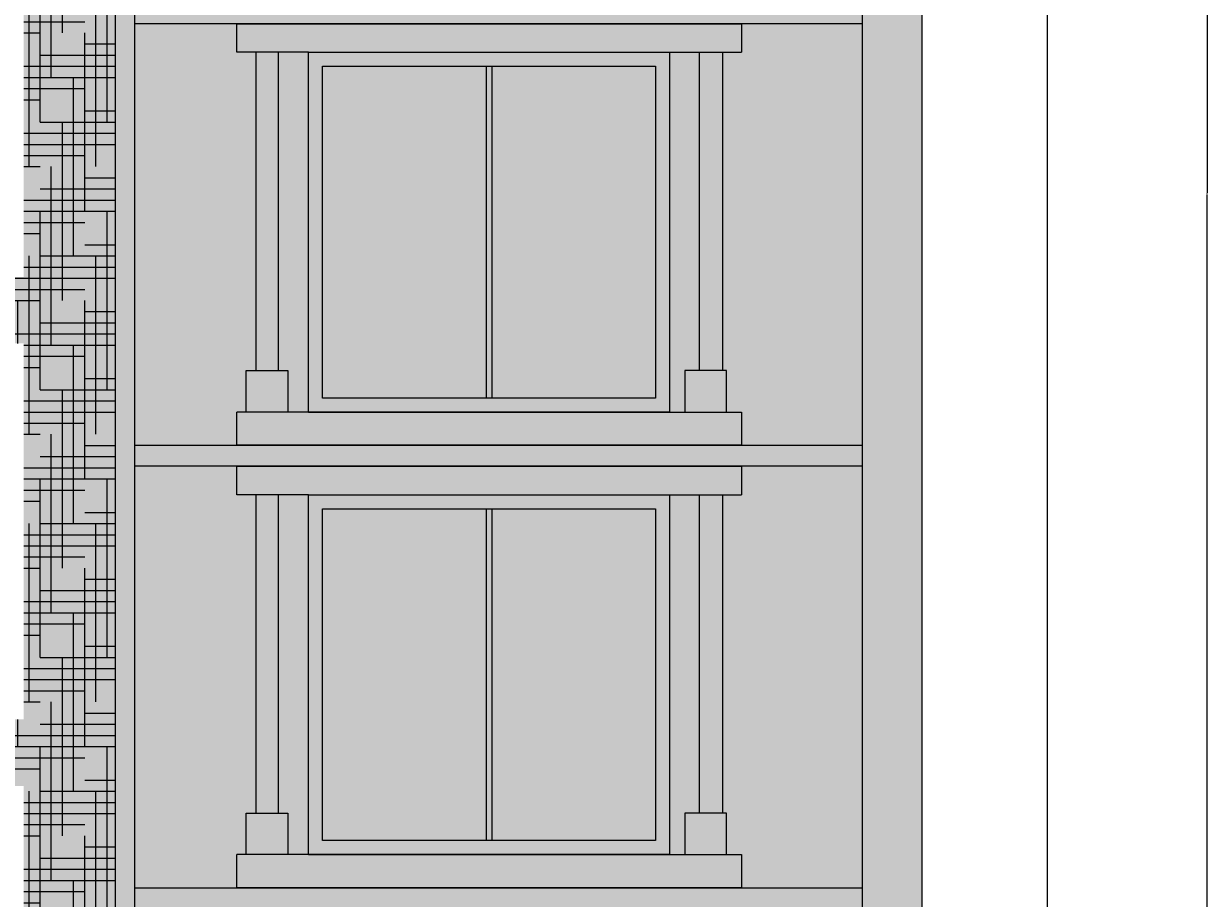
# Model space of a CAD drawing. Units: inches. Extents: x 3024 to 4744, y 1110 to 2100.
# Tile 17 of 29: x 3450 to 3787, y 1405 to 1654. Entities that reach past the tile are written whole.
import ezdxf

# ---------------------------------------------------------------- set-up
doc = ezdxf.new("R2010")
doc.units = ezdxf.units.IN
for name, color, linetype, lineweight in [('A-ANNO-DIMS', 2, 'Continuous', 18), ('A-ELEV', 7, 'Continuous', 25), ('A-ELEV-PATT', 252, 'Continuous', 13), ('A-GLAZ', 4, 'Continuous', 18)]:
    doc.layers.add(name, color=color, linetype=linetype, lineweight=lineweight)
doc.styles.get("Standard").update_dxf_attribs({"font": 'arial.ttf'})
doc.dimstyles.get("Standard").update_dxf_attribs({"dimtxt": 0.18, "dimasz": 0.18, "dimexe": 0.18, "dimexo": 0.0625, "dimgap": 0.09, "dimtad": 0, "dimtih": 1, "dimtoh": 1, "dimdec": 1, "dimzin": 0, "dimdsep": 46, "dimlunit": 3, "dimtxsty": 'Standard', "dimcen": 0.09, "dimadec": 0, "dimazin": 0, "dimtfac": 1, "dimtdec": 1, "dimtofl": 0, "dimtmove": 0, "dimatfit": 3, "dimfxl": 1, "dimtolj": 1, "dimtzin": 0, "dimarcsym": 0})

# ---------------------------------------------------------------- blocks, each defined once
blk = doc.blocks.new('WIN-BALCONY-A')
for p, q in [((3169.4, 1897.49), (3148.97, 1897.49)), ((3169.4, 1897.49), (3148.97, 1897.49)), ((3169.4, 1897.49), (3292.61, 1897.49)), ((3169.4, 1897.49), (3292.61, 1897.49)), ((3169.4, 1795.04), (3148.97, 1795.04)), ((3169.4, 1795.04), (3148.97, 1795.04)), ((3169.4, 1795.04), (3292.61, 1795.04)), ((3169.4, 1795.04), (3292.61, 1795.04))]:
    blk.add_line(p, q)
for points in [[(3148.97, 1897.49), (3148.97, 1905.61), (3292.61, 1905.61), (3292.61, 1897.49)], [(3148.97, 1897.49), (3148.97, 1905.61), (3292.61, 1905.61), (3292.61, 1897.49)], [(3292.61, 1795.04), (3292.61, 1785.61), (3148.97, 1785.61), (3148.97, 1795.04)], [(3292.61, 1795.04), (3292.61, 1785.61), (3148.97, 1785.61), (3148.97, 1795.04)]]:
    blk.add_lwpolyline(points)
for points in [[(3154.33, 1806.87), (3160.86, 1806.87), (3160.86, 1897.49), (3154.33, 1897.49)], [(3154.33, 1806.87), (3160.86, 1806.87), (3160.86, 1897.49), (3154.33, 1897.49)], [(3272.18, 1795.04), (3169.4, 1795.04), (3169.4, 1897.49), (3272.18, 1897.49)], [(3272.18, 1795.04), (3169.4, 1795.04), (3169.4, 1897.49), (3272.18, 1897.49)], [(3287.25, 1806.87), (3280.72, 1806.87), (3280.72, 1897.49), (3287.25, 1897.49)], [(3287.25, 1806.87), (3280.72, 1806.87), (3280.72, 1897.49), (3287.25, 1897.49)], [(3268.18, 1799.04), (3173.4, 1799.04), (3173.4, 1893.49), (3268.18, 1893.49)], [(3268.18, 1799.04), (3173.4, 1799.04), (3173.4, 1893.49), (3268.18, 1893.49)], [(3220.05, 1893.49), (3221.52, 1893.49), (3221.52, 1799.04), (3220.05, 1799.04)], [(3220.05, 1893.49), (3221.52, 1893.49), (3221.52, 1799.04), (3220.05, 1799.04)], [(3163.53, 1795.04), (3151.66, 1795.04), (3151.66, 1806.87), (3163.53, 1806.87)], [(3163.53, 1795.04), (3151.66, 1795.04), (3151.66, 1806.87), (3163.53, 1806.87)], [(3276.51, 1795.04), (3288.38, 1795.04), (3288.38, 1806.87), (3276.51, 1806.87)], [(3276.51, 1795.04), (3288.38, 1795.04), (3288.38, 1806.87), (3276.51, 1806.87)]]:
    blk.add_lwpolyline(points, close=True)
blk = doc.blocks.new('*D64')
at = {"layer": 'A-ANNO-DIMS', "color": 0, "lineweight": -2, "transparency": 16777216}
for p, q in [((3069.79, 1241.5), (3069.79, 2100.44)), ((3069.97, 2100.26), (3405.08, 2100.26)), ((3740.97, 2100.26), (3405.87, 2100.26)), ((3741.15, 1241.5), (3741.15, 2100.44))]:
    blk.add_line(p, q, dxfattribs=at)
at = {"layer": 'A-ANNO-DIMS', "color": 0, "transparency": 16777216}
for points in [[(3069.97, 2100.29), (3069.97, 2100.23), (3069.79, 2100.26)], [(3740.97, 2100.29), (3740.97, 2100.23), (3741.15, 2100.26)]]:
    blk.add_solid(points, dxfattribs=at)
at = {"layer": 'Defpoints', "color": 0, "transparency": 16777216}
for p in [(3741.15, 2100.26), (3069.79, 1241.43), (3741.15, 1241.43)]:
    blk.add_point(p, dxfattribs=at)
at = {"layer": 'A-ANNO-DIMS', "color": 0, "transparency": 16777216, "insert": (3405.47, 2100.26), "char_height": 0.18, "attachment_point": 5}
blk.add_mtext('\\A1;671.4', dxfattribs=at)
blk = doc.blocks.new('*D75')
at = {"layer": 'A-ANNO-DIMS', "color": 0, "lineweight": -2, "transparency": 16777216}
for p, q in [((3491.89, 2054.76), (3786.83, 2054.76)), ((3786.65, 2054.58), (3786.65, 1605.37)), ((3786.65, 1155.79), (3786.65, 1605)), ((3741.21, 1155.61), (3786.83, 1155.61))]:
    blk.add_line(p, q, dxfattribs=at)
at = {"layer": 'A-ANNO-DIMS', "color": 0, "transparency": 16777216}
for points in [[(3786.62, 2054.58), (3786.68, 2054.58), (3786.65, 2054.76)], [(3786.62, 1155.79), (3786.68, 1155.79), (3786.65, 1155.61)]]:
    blk.add_solid(points, dxfattribs=at)
at = {"layer": 'Defpoints', "color": 0, "transparency": 16777216}
for p in [(3491.83, 2054.76), (3786.65, 2054.76), (3741.15, 1155.61)]:
    blk.add_point(p, dxfattribs=at)
at = {"layer": 'A-ANNO-DIMS', "color": 0, "transparency": 16777216, "insert": (3786.65, 1605.18), "char_height": 0.18, "attachment_point": 5}
blk.add_mtext('\\A1;899.1', dxfattribs=at)

msp = doc.modelspace()

# ---------------------------------------------------------------- hatches: boundary and pattern name
at = {"layer": 'A-ELEV-PATT'}
h = msp.add_hatch(color=256, dxfattribs=at)
h.dxf.hatch_style = 1
h.paths.add_polyline_path([(3491.8271, 2054.7584), (3320.5658, 2054.7584), (3320.5658, 2043.5286), (3491.8271, 2043.5286)])
h.paths.add_polyline_path([(3292.6051, 1905.6112), (3148.9694, 1905.6112), (3148.9694, 1897.4879), (3169.3964, 1897.4879), (3292.6051, 1897.4879)])
h.paths.add_polyline_path([(3292.6051, 1795.0431), (3169.3964, 1795.0431), (3148.9694, 1795.0431), (3148.9694, 1785.6112), (3292.6051, 1785.6112)])
h.paths.add_polyline_path([(3292.6051, 1779.6112), (3148.9694, 1779.6112), (3148.9694, 1771.4879), (3169.3964, 1771.4879), (3292.6051, 1771.4879)])
h.paths.add_polyline_path([(3292.6051, 1669.0431), (3169.3964, 1669.0431), (3148.9694, 1669.0431), (3148.9694, 1659.6112), (3292.6051, 1659.6112)])
h.paths.add_polyline_path([(3292.6051, 1653.6112), (3148.9694, 1653.6112), (3148.9694, 1645.4879), (3169.3964, 1645.4879), (3292.6051, 1645.4879)])
h.paths.add_polyline_path([(3292.6051, 1543.0431), (3169.3964, 1543.0431), (3148.9694, 1543.0431), (3148.9694, 1533.6112), (3292.6051, 1533.6112)])
h.paths.add_polyline_path([(3292.6051, 1527.6112), (3148.9694, 1527.6112), (3148.9694, 1519.4879), (3169.3964, 1519.4879), (3292.6051, 1519.4879)])
h.paths.add_polyline_path([(3292.6051, 1401.6112), (3148.9694, 1401.6112), (3148.9694, 1393.4879), (3169.3964, 1393.4879), (3292.6051, 1393.4879)])
h.paths.add_polyline_path([(3292.6051, 1417.0431), (3169.3964, 1417.0431), (3148.9694, 1417.0431), (3148.9694, 1407.6112), (3292.6051, 1407.6112)])
h.paths.add_polyline_path([(3292.6051, 1291.0431), (3169.3964, 1291.0431), (3148.9694, 1291.0431), (3148.9694, 1281.6112), (3292.6051, 1281.6112)])
h.paths.add_polyline_path([(3654.037, 1165.0431), (3530.8283, 1165.0431), (3510.4013, 1165.0431), (3510.4013, 1155.6112), (3654.037, 1155.6112)])
h.paths.add_polyline_path([(3654.037, 1275.6112), (3510.4013, 1275.6112), (3510.4013, 1267.4879), (3530.8283, 1267.4879), (3654.037, 1267.4879)])
h.paths.add_polyline_path([(3654.037, 1291.0431), (3530.8283, 1291.0431), (3510.4013, 1291.0431), (3510.4013, 1281.6112), (3654.037, 1281.6112)])
h.paths.add_polyline_path([(3654.037, 1417.0431), (3530.8283, 1417.0431), (3510.4013, 1417.0431), (3510.4013, 1407.6112), (3654.037, 1407.6112)])
h.paths.add_polyline_path([(3654.037, 1401.6112), (3510.4013, 1401.6112), (3510.4013, 1393.4879), (3530.8283, 1393.4879), (3654.037, 1393.4879)])
h.paths.add_polyline_path([(3654.037, 1543.0431), (3530.8283, 1543.0431), (3510.4013, 1543.0431), (3510.4013, 1533.6112), (3654.037, 1533.6112)])
h.paths.add_polyline_path([(3654.037, 1527.6112), (3510.4013, 1527.6112), (3510.4013, 1519.4879), (3530.8283, 1519.4879), (3654.037, 1519.4879)])
h.paths.add_polyline_path([(3654.037, 1653.6112), (3510.4013, 1653.6112), (3510.4013, 1645.4879), (3530.8283, 1645.4879), (3654.037, 1645.4879)])
h.paths.add_polyline_path([(3654.037, 1669.0431), (3530.8283, 1669.0431), (3510.4013, 1669.0431), (3510.4013, 1659.6112), (3654.037, 1659.6112)])
h.paths.add_polyline_path([(3654.037, 1779.6112), (3510.4013, 1779.6112), (3510.4013, 1771.4879), (3530.8283, 1771.4879), (3654.037, 1771.4879)])
h.paths.add_polyline_path([(3654.037, 1795.0431), (3530.8283, 1795.0431), (3510.4013, 1795.0431), (3510.4013, 1785.6112), (3654.037, 1785.6112)])
h.paths.add_polyline_path([(3654.037, 1905.6112), (3510.4013, 1905.6112), (3510.4013, 1897.4879), (3530.8283, 1897.4879), (3654.037, 1897.4879)])
h = msp.add_hatch(color=256, dxfattribs=at)
h.dxf.hatch_style = 1
h.paths.add_polyline_path([(3335.1044, 2043.5286), (3329.7033, 2043.5286), (3329.7033, 1155.6112), (3335.1044, 1155.6112)])
h.paths.add_polyline_path([(3481.2411, 2043.5286), (3335.1044, 2043.5286), (3335.1044, 1155.6112), (3481.2411, 1155.6112)])
h.paths.add_polyline_path([(3449.7202, 1329.5246), (3361.2242, 1329.5246), (3361.2242, 1436.6064), (3449.7202, 1436.6064)], flags=16)
h.paths.add_polyline_path([(3445.7202, 1333.5246), (3365.2242, 1333.5246), (3365.2242, 1432.6064), (3445.7202, 1432.6064)], flags=0)
h.paths.add_polyline_path([(3449.7202, 1455.5246), (3361.2242, 1455.5246), (3361.2242, 1562.6064), (3449.7202, 1562.6064)], flags=16)
h.paths.add_polyline_path([(3445.7202, 1459.5246), (3365.2242, 1459.5246), (3365.2242, 1558.6064), (3445.7202, 1558.6064)], flags=0)
h.paths.add_polyline_path([(3449.7202, 1581.5246), (3361.2242, 1581.5246), (3361.2242, 1688.6064), (3449.7202, 1688.6064)], flags=16)
h.paths.add_polyline_path([(3445.7202, 1585.5246), (3365.2242, 1585.5246), (3365.2242, 1684.6064), (3445.7202, 1684.6064)], flags=0)
h.paths.add_polyline_path([(3449.7202, 1707.5246), (3361.2242, 1707.5246), (3361.2242, 1814.6064), (3449.7202, 1814.6064)], flags=16)
h.paths.add_polyline_path([(3445.7202, 1711.5246), (3365.2242, 1711.5246), (3365.2242, 1810.6064), (3445.7202, 1810.6064)], flags=0)
h.paths.add_polyline_path([(3449.7202, 1833.5246), (3361.2242, 1833.5246), (3361.2242, 1940.6064), (3449.7202, 1940.6064)], flags=16)
h.paths.add_polyline_path([(3445.7202, 1837.5246), (3365.2242, 1837.5246), (3365.2242, 1936.6064), (3445.7202, 1936.6064)], flags=0)
h = msp.add_hatch(color=256, dxfattribs=at)
h.dxf.hatch_style = 1
h.paths.add_polyline_path([(3475.84, 2043.5286), (3335.1044, 2043.5286), (3335.1044, 1155.6112), (3475.84, 1155.6112)])
h.paths.add_polyline_path([(3449.7202, 1940.6064), (3449.7202, 1833.5246), (3361.2242, 1833.5246), (3361.2242, 1940.6064)], flags=16)
h.paths.add_polyline_path([(3445.7202, 1936.6064), (3445.7202, 1837.5246), (3365.2242, 1837.5246), (3365.2242, 1936.6064)], flags=0)
h.paths.add_polyline_path([(3449.7202, 1814.6064), (3449.7202, 1707.5246), (3361.2242, 1707.5246), (3361.2242, 1814.6064)], flags=16)
h.paths.add_polyline_path([(3445.7202, 1810.6064), (3445.7202, 1711.5246), (3365.2242, 1711.5246), (3365.2242, 1810.6064)], flags=0)
h.paths.add_polyline_path([(3449.7202, 1688.6064), (3449.7202, 1581.5246), (3361.2242, 1581.5246), (3361.2242, 1688.6064)], flags=16)
h.paths.add_polyline_path([(3445.7202, 1684.6064), (3445.7202, 1585.5246), (3365.2242, 1585.5246), (3365.2242, 1684.6064)], flags=0)
h.paths.add_polyline_path([(3449.7202, 1562.6064), (3449.7202, 1455.5246), (3361.2242, 1455.5246), (3361.2242, 1562.6064)], flags=16)
h.paths.add_polyline_path([(3445.7202, 1558.6064), (3445.7202, 1459.5246), (3365.2242, 1459.5246), (3365.2242, 1558.6064)], flags=0)
h.paths.add_polyline_path([(3449.7202, 1436.6064), (3449.7202, 1329.5246), (3361.2242, 1329.5246), (3361.2242, 1436.6064)], flags=16)
h.paths.add_polyline_path([(3445.7202, 1432.6064), (3445.7202, 1333.5246), (3365.2242, 1333.5246), (3365.2242, 1432.6064)], flags=0)
h = msp.add_hatch(dxfattribs=at)
h.set_pattern_fill('HOUND', color=256, scale=2)
h.paths.add_polyline_path([(3475.84, 2043.5286), (3335.1044, 2043.5286), (3335.1044, 1155.6112), (3475.84, 1155.6112)])
h.paths.add_polyline_path([(3449.7202, 1940.6064), (3449.7202, 1833.5246), (3361.2242, 1833.5246), (3361.2242, 1940.6064)], flags=16)
h.paths.add_polyline_path([(3445.7202, 1936.6064), (3445.7202, 1837.5246), (3365.2242, 1837.5246), (3365.2242, 1936.6064)], flags=0)
h.paths.add_polyline_path([(3449.7202, 1814.6064), (3449.7202, 1707.5246), (3361.2242, 1707.5246), (3361.2242, 1814.6064)], flags=16)
h.paths.add_polyline_path([(3445.7202, 1810.6064), (3445.7202, 1711.5246), (3365.2242, 1711.5246), (3365.2242, 1810.6064)], flags=0)
h.paths.add_polyline_path([(3449.7202, 1688.6064), (3449.7202, 1581.5246), (3361.2242, 1581.5246), (3361.2242, 1688.6064)], flags=16)
h.paths.add_polyline_path([(3445.7202, 1684.6064), (3445.7202, 1585.5246), (3365.2242, 1585.5246), (3365.2242, 1684.6064)], flags=0)
h.paths.add_polyline_path([(3449.7202, 1562.6064), (3449.7202, 1455.5246), (3361.2242, 1455.5246), (3361.2242, 1562.6064)], flags=16)
h.paths.add_polyline_path([(3445.7202, 1558.6064), (3445.7202, 1459.5246), (3365.2242, 1459.5246), (3365.2242, 1558.6064)], flags=0)
h.paths.add_polyline_path([(3449.7202, 1436.6064), (3449.7202, 1329.5246), (3361.2242, 1329.5246), (3361.2242, 1436.6064)], flags=16)
h.paths.add_polyline_path([(3445.7202, 1432.6064), (3445.7202, 1333.5246), (3365.2242, 1333.5246), (3365.2242, 1432.6064)], flags=0)
h = msp.add_hatch(color=256, dxfattribs=at)
h.dxf.hatch_style = 1
h.paths.add_polyline_path([(3705.4722, 2014.6567), (3688.5588, 2014.6567), (3481.2411, 2014.6567), (3481.2411, 2009.1664), (3688.5588, 2009.1664), (3688.5588, 1155.6112), (3705.4722, 1155.6112), (3705.4722, 1911.6112)])
h = msp.add_hatch(color=256, dxfattribs=at)
h.dxf.hatch_style = 1
h.paths.add_polyline_path([(3154.3287, 1897.4879), (3148.9694, 1897.4879), (3148.9694, 1905.6112), (3105.4722, 1905.6112), (3105.4722, 1785.6112), (3148.9694, 1785.6112), (3148.9694, 1795.0431), (3151.6604, 1795.0431), (3151.6604, 1806.8674), (3154.3287, 1806.8674)])
h.paths.add_polyline_path([(3329.7033, 1905.6112), (3292.6051, 1905.6112), (3292.6051, 1897.4879), (3287.2458, 1897.4879), (3287.2458, 1806.8674), (3288.3759, 1806.8674), (3288.3759, 1795.0431), (3292.6051, 1795.0431), (3292.6051, 1785.6112), (3329.7033, 1785.6112)])
h.paths.add_polyline_path([(3154.3287, 1771.4879), (3148.9694, 1771.4879), (3148.9694, 1779.6112), (3105.4722, 1779.6112), (3105.4722, 1659.6112), (3148.9694, 1659.6112), (3148.9694, 1669.0431), (3151.6604, 1669.0431), (3151.6604, 1680.8674), (3154.3287, 1680.8674)])
h.paths.add_polyline_path([(3329.7033, 1779.6112), (3292.6051, 1779.6112), (3292.6051, 1771.4879), (3287.2458, 1771.4879), (3287.2458, 1680.8674), (3288.3759, 1680.8674), (3288.3759, 1669.0431), (3292.6051, 1669.0431), (3292.6051, 1659.6112), (3329.7033, 1659.6112)])
h.paths.add_polyline_path([(3154.3287, 1645.4879), (3148.9694, 1645.4879), (3148.9694, 1653.6112), (3105.4722, 1653.6112), (3105.4722, 1533.6112), (3148.9694, 1533.6112), (3148.9694, 1543.0431), (3151.6604, 1543.0431), (3151.6604, 1554.8674), (3154.3287, 1554.8674)])
h.paths.add_polyline_path([(3329.7033, 1653.6112), (3292.6051, 1653.6112), (3292.6051, 1645.4879), (3287.2458, 1645.4879), (3287.2458, 1554.8674), (3288.3759, 1554.8674), (3288.3759, 1543.0431), (3292.6051, 1543.0431), (3292.6051, 1533.6112), (3329.7033, 1533.6112)])
h.paths.add_polyline_path([(3329.7033, 1527.6112), (3292.6051, 1527.6112), (3292.6051, 1519.4879), (3287.2458, 1519.4879), (3287.2458, 1428.8674), (3288.3759, 1428.8674), (3288.3759, 1417.0431), (3292.6051, 1417.0431), (3292.6051, 1407.6112), (3329.7033, 1407.6112)])
h.paths.add_polyline_path([(3329.7033, 1401.6112), (3292.6051, 1401.6112), (3292.6051, 1393.4879), (3287.2458, 1393.4879), (3287.2458, 1302.8674), (3288.3759, 1302.8674), (3288.3759, 1291.0431), (3292.6051, 1291.0431), (3292.6051, 1281.6112), (3329.7033, 1281.6112)])
h.paths.add_polyline_path([(3154.3287, 1393.4879), (3148.9694, 1393.4879), (3148.9694, 1401.6112), (3105.4722, 1401.6112), (3105.4722, 1281.6112), (3148.9694, 1281.6112), (3148.9694, 1291.0431), (3151.6604, 1291.0431), (3151.6604, 1302.8674), (3154.3287, 1302.8674)])
h.paths.add_polyline_path([(3154.3287, 1519.4879), (3148.9694, 1519.4879), (3148.9694, 1527.6112), (3105.4722, 1527.6112), (3105.4722, 1407.6112), (3148.9694, 1407.6112), (3148.9694, 1417.0431), (3151.6604, 1417.0431), (3151.6604, 1428.8674), (3154.3287, 1428.8674)])
h.paths.add_polyline_path([(3515.7606, 1897.4879), (3510.4013, 1897.4879), (3510.4013, 1905.6112), (3481.2411, 1905.6112), (3481.2411, 1785.6112), (3510.4013, 1785.6112), (3510.4013, 1795.0431), (3513.0923, 1795.0431), (3513.0923, 1806.8674), (3515.7606, 1806.8674)])
h.paths.add_polyline_path([(3688.5588, 1905.6112), (3654.037, 1905.6112), (3654.037, 1897.4879), (3648.6777, 1897.4879), (3648.6777, 1806.8674), (3649.8078, 1806.8674), (3649.8078, 1795.0431), (3654.037, 1795.0431), (3654.037, 1785.6112), (3688.5588, 1785.6112)])
h.paths.add_polyline_path([(3515.7606, 1771.4879), (3510.4013, 1771.4879), (3510.4013, 1779.6112), (3481.2411, 1779.6112), (3481.2411, 1659.6112), (3510.4013, 1659.6112), (3510.4013, 1669.0431), (3513.0923, 1669.0431), (3513.0923, 1680.8674), (3515.7606, 1680.8674)])
h.paths.add_polyline_path([(3688.5588, 1779.6112), (3654.037, 1779.6112), (3654.037, 1771.4879), (3648.6777, 1771.4879), (3648.6777, 1680.8674), (3649.8078, 1680.8674), (3649.8078, 1669.0431), (3654.037, 1669.0431), (3654.037, 1659.6112), (3688.5588, 1659.6112)])
h.paths.add_polyline_path([(3515.7606, 1645.4879), (3510.4013, 1645.4879), (3510.4013, 1653.6112), (3481.2411, 1653.6112), (3481.2411, 1533.6112), (3510.4013, 1533.6112), (3510.4013, 1543.0431), (3513.0923, 1543.0431), (3513.0923, 1554.8674), (3515.7606, 1554.8674)])
h.paths.add_polyline_path([(3688.5588, 1653.6112), (3654.037, 1653.6112), (3654.037, 1645.4879), (3648.6777, 1645.4879), (3648.6777, 1554.8674), (3649.8078, 1554.8674), (3649.8078, 1543.0431), (3654.037, 1543.0431), (3654.037, 1533.6112), (3688.5588, 1533.6112)])
h.paths.add_polyline_path([(3515.7606, 1519.4879), (3510.4013, 1519.4879), (3510.4013, 1527.6112), (3481.2411, 1527.6112), (3481.2411, 1407.6112), (3510.4013, 1407.6112), (3510.4013, 1417.0431), (3513.0923, 1417.0431), (3513.0923, 1428.8674), (3515.7606, 1428.8674)])
h.paths.add_polyline_path([(3688.5588, 1527.6112), (3654.037, 1527.6112), (3654.037, 1519.4879), (3648.6777, 1519.4879), (3648.6777, 1428.8674), (3649.8078, 1428.8674), (3649.8078, 1417.0431), (3654.037, 1417.0431), (3654.037, 1407.6112), (3688.5588, 1407.6112)])
h.paths.add_polyline_path([(3515.7606, 1393.4879), (3510.4013, 1393.4879), (3510.4013, 1401.6112), (3481.2411, 1401.6112), (3481.2411, 1281.6112), (3510.4013, 1281.6112), (3510.4013, 1291.0431), (3513.0923, 1291.0431), (3513.0923, 1302.8674), (3515.7606, 1302.8674)])
h.paths.add_polyline_path([(3688.5588, 1401.6112), (3654.037, 1401.6112), (3654.037, 1393.4879), (3648.6777, 1393.4879), (3648.6777, 1302.8674), (3649.8078, 1302.8674), (3649.8078, 1291.0431), (3654.037, 1291.0431), (3654.037, 1281.6112), (3688.5588, 1281.6112)])
h.paths.add_polyline_path([(3515.7606, 1267.4879), (3510.4013, 1267.4879), (3510.4013, 1275.6112), (3481.2411, 1275.6112), (3481.2411, 1155.6112), (3510.4013, 1155.6112), (3510.4013, 1165.0431), (3513.0923, 1165.0431), (3513.0923, 1176.8674), (3515.7606, 1176.8674)])
h.paths.add_polyline_path([(3688.5588, 1275.6112), (3654.037, 1275.6112), (3654.037, 1267.4879), (3648.6777, 1267.4879), (3648.6777, 1176.8674), (3649.8078, 1176.8674), (3649.8078, 1165.0431), (3654.037, 1165.0431), (3654.037, 1155.6112), (3688.5588, 1155.6112)])
h.paths.add_polyline_path([(3112.3838, 1275.6112), (3105.4722, 1275.6112), (3105.4722, 1171.0239), (3112.3838, 1171.0239)])
h = msp.add_hatch(color=256, dxfattribs=at)
h.dxf.hatch_style = 1
h.paths.add_polyline_path([(3160.8586, 1897.4879), (3154.3287, 1897.4879), (3154.3287, 1806.8674), (3160.8586, 1806.8674)])
h.paths.add_polyline_path([(3287.2458, 1897.4879), (3280.716, 1897.4879), (3280.716, 1806.8674), (3287.2458, 1806.8674)])
h.paths.add_polyline_path([(3160.8586, 1771.4879), (3154.3287, 1771.4879), (3154.3287, 1680.8674), (3160.8586, 1680.8674)])
h.paths.add_polyline_path([(3287.2458, 1771.4879), (3280.716, 1771.4879), (3280.716, 1680.8674), (3287.2458, 1680.8674)])
h.paths.add_polyline_path([(3160.8586, 1645.4879), (3154.3287, 1645.4879), (3154.3287, 1554.8674), (3160.8586, 1554.8674)])
h.paths.add_polyline_path([(3287.2458, 1645.4879), (3280.716, 1645.4879), (3280.716, 1554.8674), (3287.2458, 1554.8674)])
h.paths.add_polyline_path([(3160.8586, 1519.4879), (3154.3287, 1519.4879), (3154.3287, 1428.8674), (3160.8586, 1428.8674)])
h.paths.add_polyline_path([(3287.2458, 1519.4879), (3280.716, 1519.4879), (3280.716, 1428.8674), (3287.2458, 1428.8674)])
h.paths.add_polyline_path([(3160.8586, 1393.4879), (3154.3287, 1393.4879), (3154.3287, 1302.8674), (3160.8586, 1302.8674)])
h.paths.add_polyline_path([(3287.2458, 1393.4879), (3280.716, 1393.4879), (3280.716, 1302.8674), (3287.2458, 1302.8674)])
h.paths.add_polyline_path([(3648.6777, 1267.4879), (3642.1479, 1267.4879), (3642.1479, 1176.8674), (3648.6777, 1176.8674)])
h.paths.add_polyline_path([(3522.2905, 1267.4879), (3515.7606, 1267.4879), (3515.7606, 1176.8674), (3522.2905, 1176.8674)])
h.paths.add_polyline_path([(3522.2905, 1393.4879), (3515.7606, 1393.4879), (3515.7606, 1302.8674), (3522.2905, 1302.8674)])
h.paths.add_polyline_path([(3648.6777, 1393.4879), (3642.1479, 1393.4879), (3642.1479, 1302.8674), (3648.6777, 1302.8674)])
h.paths.add_polyline_path([(3522.2905, 1519.4879), (3515.7606, 1519.4879), (3515.7606, 1428.8674), (3522.2905, 1428.8674)])
h.paths.add_polyline_path([(3648.6777, 1519.4879), (3642.1479, 1519.4879), (3642.1479, 1428.8674), (3648.6777, 1428.8674)])
h.paths.add_polyline_path([(3522.2905, 1645.4879), (3515.7606, 1645.4879), (3515.7606, 1554.8674), (3522.2905, 1554.8674)])
h.paths.add_polyline_path([(3522.2905, 1771.4879), (3515.7606, 1771.4879), (3515.7606, 1680.8674), (3522.2905, 1680.8674)])
h.paths.add_polyline_path([(3648.6777, 1645.4879), (3642.1479, 1645.4879), (3642.1479, 1554.8674), (3648.6777, 1554.8674)])
h.paths.add_polyline_path([(3648.6777, 1771.4879), (3642.1479, 1771.4879), (3642.1479, 1680.8674), (3648.6777, 1680.8674)])
h.paths.add_polyline_path([(3648.6777, 1897.4879), (3642.1479, 1897.4879), (3642.1479, 1806.8674), (3648.6777, 1806.8674)])
h.paths.add_polyline_path([(3522.2905, 1897.4879), (3515.7606, 1897.4879), (3515.7606, 1806.8674), (3522.2905, 1806.8674)])
h = msp.add_hatch(color=256, dxfattribs=at)
h.dxf.hatch_style = 1
h.paths.add_polyline_path([(3169.3964, 1897.4879), (3160.8586, 1897.4879), (3160.8586, 1806.8674), (3163.5269, 1806.8674), (3163.5269, 1795.0431), (3169.3964, 1795.0431)])
h.paths.add_polyline_path([(3280.716, 1897.4879), (3272.1781, 1897.4879), (3272.1781, 1795.0431), (3276.5094, 1795.0431), (3276.5094, 1806.8674), (3280.716, 1806.8674)])
h.paths.add_polyline_path([(3280.716, 1771.4879), (3272.1781, 1771.4879), (3272.1781, 1669.0431), (3276.5094, 1669.0431), (3276.5094, 1680.8674), (3280.716, 1680.8674)])
h.paths.add_polyline_path([(3169.3964, 1771.4879), (3160.8586, 1771.4879), (3160.8586, 1680.8674), (3163.5269, 1680.8674), (3163.5269, 1669.0431), (3169.3964, 1669.0431)])
h.paths.add_polyline_path([(3169.3964, 1645.4879), (3160.8586, 1645.4879), (3160.8586, 1554.8674), (3163.5269, 1554.8674), (3163.5269, 1543.0431), (3169.3964, 1543.0431)])
h.paths.add_polyline_path([(3280.716, 1645.4879), (3272.1781, 1645.4879), (3272.1781, 1543.0431), (3276.5094, 1543.0431), (3276.5094, 1554.8674), (3280.716, 1554.8674)])
h.paths.add_polyline_path([(3169.3964, 1519.4879), (3160.8586, 1519.4879), (3160.8586, 1428.8674), (3163.5269, 1428.8674), (3163.5269, 1417.0431), (3169.3964, 1417.0431)])
h.paths.add_polyline_path([(3280.716, 1519.4879), (3272.1781, 1519.4879), (3272.1781, 1417.0431), (3276.5094, 1417.0431), (3276.5094, 1428.8674), (3280.716, 1428.8674)])
h.paths.add_polyline_path([(3169.3964, 1393.4879), (3160.8586, 1393.4879), (3160.8586, 1302.8674), (3163.5269, 1302.8674), (3163.5269, 1291.0431), (3169.3964, 1291.0431)])
h.paths.add_polyline_path([(3280.716, 1393.4879), (3272.1781, 1393.4879), (3272.1781, 1291.0431), (3276.5094, 1291.0431), (3276.5094, 1302.8674), (3280.716, 1302.8674)])
h.paths.add_polyline_path([(3642.1479, 1267.4879), (3633.61, 1267.4879), (3633.61, 1165.0431), (3637.9413, 1165.0431), (3637.9413, 1176.8674), (3642.1479, 1176.8674)])
h.paths.add_polyline_path([(3530.8283, 1267.4879), (3522.2905, 1267.4879), (3522.2905, 1176.8674), (3524.9588, 1176.8674), (3524.9588, 1165.0431), (3530.8283, 1165.0431)])
h.paths.add_polyline_path([(3642.1479, 1393.4879), (3633.61, 1393.4879), (3633.61, 1291.0431), (3637.9413, 1291.0431), (3637.9413, 1302.8674), (3642.1479, 1302.8674)])
h.paths.add_polyline_path([(3530.8283, 1393.4879), (3522.2905, 1393.4879), (3522.2905, 1302.8674), (3524.9588, 1302.8674), (3524.9588, 1291.0431), (3530.8283, 1291.0431)])
h.paths.add_polyline_path([(3530.8283, 1519.4879), (3522.2905, 1519.4879), (3522.2905, 1428.8674), (3524.9588, 1428.8674), (3524.9588, 1417.0431), (3530.8283, 1417.0431)])
h.paths.add_polyline_path([(3642.1479, 1519.4879), (3633.61, 1519.4879), (3633.61, 1417.0431), (3637.9413, 1417.0431), (3637.9413, 1428.8674), (3642.1479, 1428.8674)])
h.paths.add_polyline_path([(3530.8283, 1645.4879), (3522.2905, 1645.4879), (3522.2905, 1554.8674), (3524.9588, 1554.8674), (3524.9588, 1543.0431), (3530.8283, 1543.0431)])
h.paths.add_polyline_path([(3642.1479, 1645.4879), (3633.61, 1645.4879), (3633.61, 1543.0431), (3637.9413, 1543.0431), (3637.9413, 1554.8674), (3642.1479, 1554.8674)])
h.paths.add_polyline_path([(3642.1479, 1771.4879), (3633.61, 1771.4879), (3633.61, 1669.0431), (3637.9413, 1669.0431), (3637.9413, 1680.8674), (3642.1479, 1680.8674)])
h.paths.add_polyline_path([(3530.8283, 1771.4879), (3522.2905, 1771.4879), (3522.2905, 1680.8674), (3524.9588, 1680.8674), (3524.9588, 1669.0431), (3530.8283, 1669.0431)])
h.paths.add_polyline_path([(3530.8283, 1897.4879), (3522.2905, 1897.4879), (3522.2905, 1806.8674), (3524.9588, 1806.8674), (3524.9588, 1795.0431), (3530.8283, 1795.0431)])
h.paths.add_polyline_path([(3642.1479, 1897.4879), (3633.61, 1897.4879), (3633.61, 1795.0431), (3637.9413, 1795.0431), (3637.9413, 1806.8674), (3642.1479, 1806.8674)])
h = msp.add_hatch(color=256, dxfattribs=at)
h.dxf.hatch_style = 1
h.paths.add_polyline_path([(3220.0505, 1893.4879), (3173.3964, 1893.4879), (3173.3964, 1799.0431), (3220.0505, 1799.0431)])
h.paths.add_polyline_path([(3268.1781, 1893.4879), (3221.5241, 1893.4879), (3221.5241, 1799.0431), (3268.1781, 1799.0431)])
h.paths.add_polyline_path([(3581.4824, 1893.4879), (3534.8283, 1893.4879), (3534.8283, 1799.0431), (3581.4824, 1799.0431)])
h.paths.add_polyline_path([(3629.61, 1893.4879), (3582.956, 1893.4879), (3582.956, 1799.0431), (3629.61, 1799.0431)])
h.paths.add_polyline_path([(3581.4824, 1767.4879), (3534.8283, 1767.4879), (3534.8283, 1673.0431), (3581.4824, 1673.0431)])
h.paths.add_polyline_path([(3629.61, 1767.4879), (3582.956, 1767.4879), (3582.956, 1673.0431), (3629.61, 1673.0431)])
h.paths.add_polyline_path([(3581.4824, 1641.4879), (3534.8283, 1641.4879), (3534.8283, 1547.0431), (3581.4824, 1547.0431)])
h.paths.add_polyline_path([(3629.61, 1641.4879), (3582.956, 1641.4879), (3582.956, 1547.0431), (3629.61, 1547.0431)])
h.paths.add_polyline_path([(3629.61, 1515.4879), (3582.956, 1515.4879), (3582.956, 1421.0431), (3629.61, 1421.0431)])
h.paths.add_polyline_path([(3581.4824, 1515.4879), (3534.8283, 1515.4879), (3534.8283, 1421.0431), (3581.4824, 1421.0431)])
h.paths.add_polyline_path([(3629.61, 1389.4879), (3582.956, 1389.4879), (3582.956, 1295.0431), (3629.61, 1295.0431)])
h.paths.add_polyline_path([(3581.4824, 1389.4879), (3534.8283, 1389.4879), (3534.8283, 1295.0431), (3581.4824, 1295.0431)])
h.paths.add_polyline_path([(3629.61, 1263.4879), (3582.956, 1263.4879), (3582.956, 1169.0431), (3629.61, 1169.0431)])
h.paths.add_polyline_path([(3581.4824, 1263.4879), (3534.8283, 1263.4879), (3534.8283, 1169.0431), (3581.4824, 1169.0431)])
h.paths.add_polyline_path([(3220.0505, 1389.4879), (3173.3964, 1389.4879), (3173.3964, 1295.0431), (3220.0505, 1295.0431)])
h.paths.add_polyline_path([(3268.1781, 1389.4879), (3221.5241, 1389.4879), (3221.5241, 1295.0431), (3268.1781, 1295.0431)])
h.paths.add_polyline_path([(3220.0505, 1515.4879), (3173.3964, 1515.4879), (3173.3964, 1421.0431), (3220.0505, 1421.0431)])
h.paths.add_polyline_path([(3268.1781, 1515.4879), (3221.5241, 1515.4879), (3221.5241, 1421.0431), (3268.1781, 1421.0431)])
h.paths.add_polyline_path([(3220.0505, 1767.4879), (3173.3964, 1767.4879), (3173.3964, 1673.0431), (3220.0505, 1673.0431)])
h.paths.add_polyline_path([(3268.1781, 1767.4879), (3221.5241, 1767.4879), (3221.5241, 1673.0431), (3268.1781, 1673.0431)])
h.paths.add_polyline_path([(3220.0505, 1641.4879), (3173.3964, 1641.4879), (3173.3964, 1547.0431), (3220.0505, 1547.0431)])
h.paths.add_polyline_path([(3268.1781, 1641.4879), (3221.5241, 1641.4879), (3221.5241, 1547.0431), (3268.1781, 1547.0431)])
h = msp.add_hatch(color=256, dxfattribs=at)
h.dxf.hatch_style = 1
h.paths.add_polyline_path([(3163.5269, 1302.8674), (3151.6604, 1302.8674), (3151.6604, 1291.0431), (3163.5269, 1291.0431)])
h.paths.add_polyline_path([(3288.3759, 1302.8674), (3276.5094, 1302.8674), (3276.5094, 1291.0431), (3288.3759, 1291.0431)])
h.paths.add_polyline_path([(3288.3759, 1428.8674), (3276.5094, 1428.8674), (3276.5094, 1417.0431), (3288.3759, 1417.0431)])
h.paths.add_polyline_path([(3163.5269, 1428.8674), (3151.6604, 1428.8674), (3151.6604, 1417.0431), (3163.5269, 1417.0431)])
h.paths.add_polyline_path([(3163.5269, 1554.8674), (3151.6604, 1554.8674), (3151.6604, 1543.0431), (3163.5269, 1543.0431)])
h.paths.add_polyline_path([(3288.3759, 1554.8674), (3276.5094, 1554.8674), (3276.5094, 1543.0431), (3288.3759, 1543.0431)])
h.paths.add_polyline_path([(3163.5269, 1680.8674), (3151.6604, 1680.8674), (3151.6604, 1669.0431), (3163.5269, 1669.0431)])
h.paths.add_polyline_path([(3288.3759, 1680.8674), (3276.5094, 1680.8674), (3276.5094, 1669.0431), (3288.3759, 1669.0431)])
h.paths.add_polyline_path([(3163.5269, 1806.8674), (3151.6604, 1806.8674), (3151.6604, 1795.0431), (3163.5269, 1795.0431)])
h.paths.add_polyline_path([(3288.3759, 1806.8674), (3276.5094, 1806.8674), (3276.5094, 1795.0431), (3288.3759, 1795.0431)])
h.paths.add_polyline_path([(3524.9588, 1806.8674), (3513.0923, 1806.8674), (3513.0923, 1795.0431), (3524.9588, 1795.0431)])
h.paths.add_polyline_path([(3649.8078, 1806.8674), (3637.9413, 1806.8674), (3637.9413, 1795.0431), (3649.8078, 1795.0431)])
h.paths.add_polyline_path([(3524.9588, 1680.8674), (3513.0923, 1680.8674), (3513.0923, 1669.0431), (3524.9588, 1669.0431)])
h.paths.add_polyline_path([(3649.8078, 1680.8674), (3637.9413, 1680.8674), (3637.9413, 1669.0431), (3649.8078, 1669.0431)])
h.paths.add_polyline_path([(3524.9588, 1554.8674), (3513.0923, 1554.8674), (3513.0923, 1543.0431), (3524.9588, 1543.0431)])
h.paths.add_polyline_path([(3649.8078, 1554.8674), (3637.9413, 1554.8674), (3637.9413, 1543.0431), (3649.8078, 1543.0431)])
h.paths.add_polyline_path([(3524.9588, 1428.8674), (3513.0923, 1428.8674), (3513.0923, 1417.0431), (3524.9588, 1417.0431)])
h.paths.add_polyline_path([(3649.8078, 1428.8674), (3637.9413, 1428.8674), (3637.9413, 1417.0431), (3649.8078, 1417.0431)])
h.paths.add_polyline_path([(3524.9588, 1302.8674), (3513.0923, 1302.8674), (3513.0923, 1291.0431), (3524.9588, 1291.0431)])
h.paths.add_polyline_path([(3649.8078, 1302.8674), (3637.9413, 1302.8674), (3637.9413, 1291.0431), (3649.8078, 1291.0431)])
h.paths.add_polyline_path([(3524.9588, 1176.8674), (3513.0923, 1176.8674), (3513.0923, 1165.0431), (3524.9588, 1165.0431)])
h.paths.add_polyline_path([(3649.8078, 1176.8674), (3637.9413, 1176.8674), (3637.9413, 1165.0431), (3649.8078, 1165.0431)])
h = msp.add_hatch(color=256, dxfattribs=at)
h.dxf.hatch_style = 1
h.paths.add_polyline_path([(3688.5588, 1785.6112), (3481.2411, 1785.6112), (3481.2411, 1779.6112), (3688.5588, 1779.6112)])
h.paths.add_polyline_path([(3688.5588, 1659.6112), (3481.2411, 1659.6112), (3481.2411, 1653.6112), (3688.5588, 1653.6112)])
h.paths.add_polyline_path([(3688.5588, 1533.6112), (3481.2411, 1533.6112), (3481.2411, 1527.6112), (3688.5588, 1527.6112)])
h.paths.add_polyline_path([(3688.5588, 1407.6112), (3481.2411, 1407.6112), (3481.2411, 1401.6112), (3688.5588, 1401.6112)])
h.paths.add_polyline_path([(3688.5588, 1281.6112), (3481.2411, 1281.6112), (3481.2411, 1275.6112), (3688.5588, 1275.6112)])
h = msp.add_hatch(color=256, dxfattribs=at)
h.dxf.hatch_style = 1
h.paths.add_polyline_path([(3582.956, 1767.4879), (3581.4824, 1767.4879), (3581.4824, 1673.0431), (3582.956, 1673.0431)], flags=0)
h.paths.add_polyline_path([(3582.956, 1767.4879), (3582.956, 1673.0431), (3581.4824, 1673.0431), (3581.4824, 1767.4879)], flags=0)
h.paths.add_polyline_path([(3582.956, 1641.4879), (3581.4824, 1641.4879), (3581.4824, 1547.0431), (3582.956, 1547.0431)])
h = msp.add_hatch(color=256, dxfattribs=at)
h.dxf.hatch_style = 1
h.paths.add_polyline_path([(3582.956, 1641.4879), (3581.4824, 1641.4879), (3581.4824, 1547.0431), (3582.956, 1547.0431)], flags=0)
h.paths.add_polyline_path([(3633.61, 1645.4879), (3530.8283, 1645.4879), (3530.8283, 1543.0431), (3633.61, 1543.0431)])
h.paths.add_polyline_path([(3629.61, 1641.4879), (3629.61, 1547.0431), (3534.8283, 1547.0431), (3534.8283, 1641.4879)], flags=16)
h.paths.add_polyline_path([(3582.956, 1641.4879), (3582.956, 1547.0431), (3581.4824, 1547.0431), (3581.4824, 1641.4879)], flags=0)
h = msp.add_hatch(color=256, dxfattribs=at)
h.dxf.hatch_style = 1
h.paths.add_polyline_path([(3582.956, 1641.4879), (3581.4824, 1641.4879), (3581.4824, 1547.0431), (3582.956, 1547.0431)], flags=0)
h.paths.add_polyline_path([(3582.956, 1641.4879), (3582.956, 1547.0431), (3581.4824, 1547.0431), (3581.4824, 1641.4879)], flags=0)
h.paths.add_polyline_path([(3582.956, 1515.4879), (3581.4824, 1515.4879), (3581.4824, 1421.0431), (3582.956, 1421.0431)])
h = msp.add_hatch(color=256, dxfattribs=at)
h.dxf.hatch_style = 1
h.paths.add_polyline_path([(3582.956, 1515.4879), (3581.4824, 1515.4879), (3581.4824, 1421.0431), (3582.956, 1421.0431)], flags=0)
h.paths.add_polyline_path([(3633.61, 1519.4879), (3530.8283, 1519.4879), (3530.8283, 1417.0431), (3633.61, 1417.0431)])
h.paths.add_polyline_path([(3629.61, 1515.4879), (3629.61, 1421.0431), (3534.8283, 1421.0431), (3534.8283, 1515.4879)], flags=16)
h.paths.add_polyline_path([(3582.956, 1515.4879), (3582.956, 1421.0431), (3581.4824, 1421.0431), (3581.4824, 1515.4879)], flags=0)
h = msp.add_hatch(color=256, dxfattribs=at)
h.dxf.hatch_style = 1
h.paths.add_polyline_path([(3582.956, 1515.4879), (3581.4824, 1515.4879), (3581.4824, 1421.0431), (3582.956, 1421.0431)], flags=0)
h.paths.add_polyline_path([(3582.956, 1515.4879), (3582.956, 1421.0431), (3581.4824, 1421.0431), (3581.4824, 1515.4879)], flags=0)
h.paths.add_polyline_path([(3582.956, 1389.4879), (3581.4824, 1389.4879), (3581.4824, 1295.0431), (3582.956, 1295.0431)])

# ---------------------------------------------------------------- linework, layer by layer
at = {"layer": 'A-ELEV'}
for p, q in [((3705.4722, 1155.6112), (3705.4722, 1911.6112)), ((3705.4722, 1155.6112), (3705.4722, 1911.6112)), ((3688.5588, 1653.6112), (3481.2411, 1653.6112)), ((3688.5588, 1653.6112), (3481.2411, 1653.6112)), ((3481.2411, 1533.6112), (3688.5588, 1533.6112)), ((3481.2411, 1533.6112), (3688.5588, 1533.6112)), ((3688.5588, 1527.6112), (3481.2411, 1527.6112)), ((3688.5588, 1527.6112), (3481.2411, 1527.6112)), ((3481.2411, 1407.6112), (3688.5588, 1407.6112)), ((3481.2411, 1407.6112), (3688.5588, 1407.6112))]:
    msp.add_line(p, q, dxfattribs=at)
for points in [[(3481.2411, 1155.6112), (3329.7033, 1155.6112), (3329.7033, 2043.5286), (3481.2411, 2043.5286)], [(3481.2411, 1155.6112), (3329.7033, 1155.6112), (3329.7033, 2043.5286), (3481.2411, 2043.5286)], [(3475.84, 2043.5286), (3481.2411, 2043.5286), (3481.2411, 1155.6112), (3475.84, 1155.6112)], [(3475.84, 2043.5286), (3481.2411, 2043.5286), (3481.2411, 1155.6112), (3475.84, 1155.6112)], [(3475.84, 2043.5286), (3481.2411, 2043.5286), (3481.2411, 1155.6112), (3475.84, 1155.6112)]]:
    msp.add_lwpolyline(points, close=True, dxfattribs=at)
for points in [[(3705.4722, 1155.6112), (3688.5588, 1155.6112), (3688.5588, 2014.6567), (3705.4722, 2014.6567), (3705.4722, 1905.6112)], [(3705.4722, 1155.6112), (3688.5588, 1155.6112), (3688.5588, 2009.1664)]]:
    msp.add_lwpolyline(points, dxfattribs=at)

# ---------------------------------------------------------------- block references
at = {"layer": 'A-GLAZ'}
for p in [(361.4319, -252), (361.4319, -378)]:
    msp.add_blockref('WIN-BALCONY-A', p, dxfattribs=at)

# ---------------------------------------------------------------- dimensions: what is measured, and where the dimension line sits
at = {"layer": 'A-ANNO-DIMS'}
dim = msp.add_linear_dim(base=(3741.1507, 2100.2584), p1=(3069.7937, 1241.4341), p2=(3741.1507, 1241.4341), dimstyle='Standard', override={"dimdec": 1, "dimlfac": 1, "dimrnd": 0, "dimzin": 0, "dimdsep": 46, "dimlunit": 2}, dxfattribs=at)
dim.commit()
dim.dimension.update_dxf_attribs({"geometry": '*D64', "text_midpoint": (3405.4722, 2100.2584)})
dim = msp.add_linear_dim(base=(3786.6507, 2054.7584), p1=(3741.1507, 1155.6112), p2=(3491.8271, 2054.7584), angle=90, dimstyle='Standard', override={"dimdec": 1, "dimlfac": 1, "dimrnd": 0, "dimzin": 0, "dimdsep": 46, "dimlunit": 2}, dxfattribs=at)
dim.commit()
dim.dimension.update_dxf_attribs({"geometry": '*D75', "text_midpoint": (3786.6507, 1605.1848)})

doc.saveas('drawing.dxf')
